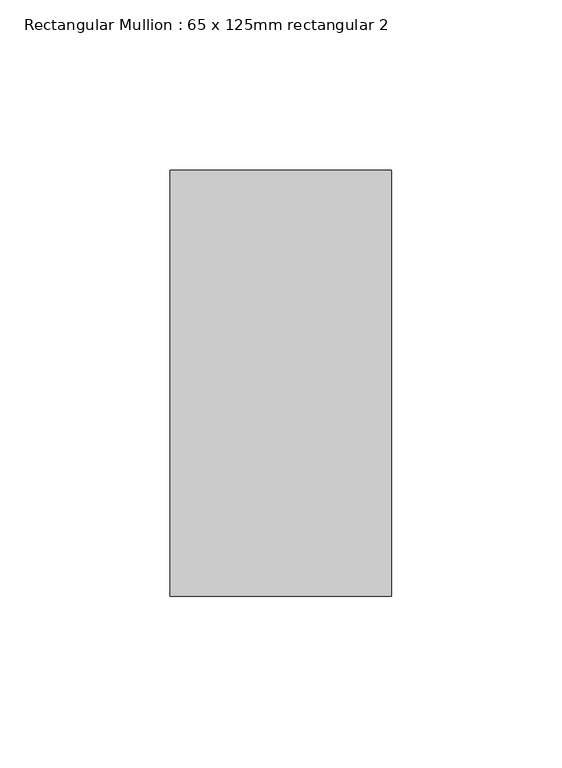
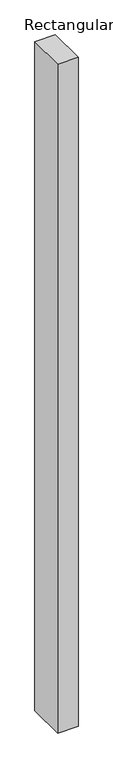
"""IFC4 building model written with IfcOpenShell, lengths in millimetres: member geometry, Rectangular Mullion : 65 x 125mm rectangular 2."""

from ifc_helpers import new_model, si_unit, frame, origin, place, context, project, spatial, polyline, outline, extrude, source, transform, mapped, element, save


def rectangular_mullion_65_x_125mm_rectangular_2_9432af82(model_context):
    return source(origin(), model_context, "Body", "SweptSolid", [
        extrude(outline(polyline([(32.5, 62.5), (32.5, -62.5), (-32.5, -62.5), (-32.5, 62.5), (32.5, 62.5)])), frame((0.0, 0.0, -2250.0), z_axis=(0.0, 0.0, 1.0), x_axis=(1.0, 0.0, 0.0)), (0.0, 0.0, 1.0), 2250.0),
    ])


if __name__ == "__main__":
    model = new_model("IFC4")
    model_context = context("Model", 3, world=origin())
    ifc_project = project(units=[si_unit("LENGTHUNIT", "METRE", prefix="MILLI")], contexts=[model_context])
    site = spatial("IfcSite", under=ifc_project)
    building = spatial("IfcBuilding", under=site)
    placement = place(None, origin())
    rectangular_mullion_65_x_125mm_rectangular_2_shape = rectangular_mullion_65_x_125mm_rectangular_2_9432af82(model_context)
    element("IfcMember", 1, ObjectType="Rectangular Mullion : 65 x 125mm rectangular 2", at=placement, inside=building, context=model_context, shape_type="MappedRepresentation", body=[
        mapped(rectangular_mullion_65_x_125mm_rectangular_2_shape, transform((0.0, 0.0, 0.0), x_axis=(1.0, 0.0, 0.0), y_axis=(0.0, 1.0, 0.0), z_axis=(0.0, 0.0, 1.0))),
    ])
    save(model, "model.ifc")

# Revit data of these elements
# Type "Rectangular Mullion : 65 x 125mm rectangular 2"
#   built-in parameter 1007304 = 0.410105 (stored number, unit not read)
#   built-in parameter 1007301 = 0.106627 (stored number, unit not read)
#   built-in parameter 1007300 = 0.106627 (stored number, unit not read)
